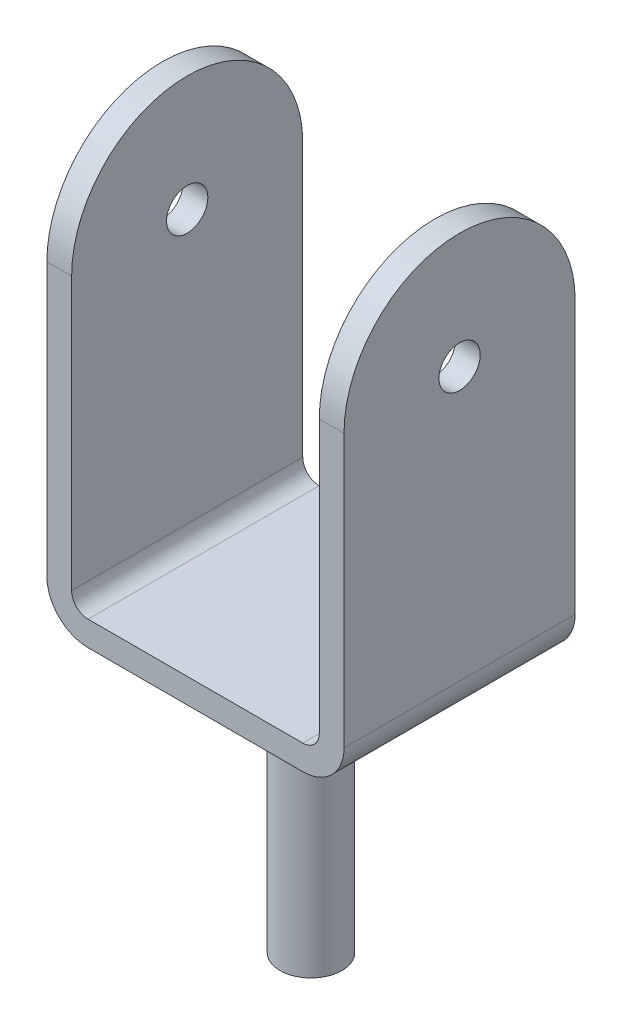
from build123d import *

# Parameters (mm, degrees)
U_CHANNEL_BODY_DEPTH     = 140
STEM_SKETCH_75_R         = 37.5
STEM_75_DEPTH            = 325
UPRIGHT_TOP_ROUNDS_R50_R = 50
CHANNEL_FILLETS_R20_R    = 20
SIDE_BOSS_SKETCH_R       = 140
SIDE_BOSS_DEPTH          = 30
PIN_HOLE_SKETCH_R        = 25
PIN_HOLES_DEPTH          = 648.765389628


with BuildPart() as part:
    # U-Channel Profile Sketch → U-Channel Body (new, symmetric)
    with BuildSketch(Plane.XY):
        Polygon((-180, 380), (-180, 0), (180, 0), (180, 380), (150, 380), (150, 30), (-150, 30), (-150, 380), align=None)
    extrude(amount=U_CHANNEL_BODY_DEPTH, both=True)

    # Stem Sketch Ø75 → Stem Ø75 (add)
    with BuildSketch(Plane.XZ):
        Circle(STEM_SKETCH_75_R)
    extrude(amount=STEM_75_DEPTH)

    # Upright Top Rounds R50
    upright_top_rounds_r50_edges = [part.edges().sort_by_distance(p)[0] for p in [
        (180, 0, 0),
        (-180, 0, 0),
    ]]
    fillet(upright_top_rounds_r50_edges, radius=UPRIGHT_TOP_ROUNDS_R50_R)

    # Channel Fillets R20
    channel_fillets_r20_edges = [part.edges().sort_by_distance(p)[0] for p in [
        (-150, 30, 0),
        (150, 30, 0),
    ]]
    fillet(channel_fillets_r20_edges, radius=CHANNEL_FILLETS_R20_R)

    # Side Boss Sketch → Side Boss (add)
    with BuildSketch(Plane(origin=(180, 0, 0), x_dir=(0, 0, -1), z_dir=(1, 0, 0))):
        with Locations((0, 380)):
            Circle(SIDE_BOSS_SKETCH_R)
    side_boss = extrude(amount=-SIDE_BOSS_DEPTH)

    # Side Boss Mirror: Side Boss across plane
    add(side_boss.mirror(Plane(origin=(0, 0, 0), x_dir=(0, 0, 1), z_dir=(1, 0, 0))))

    # Pin Hole Sketch → Pin Holes (cut, through all)
    with BuildSketch(Plane.ZY.offset(180)):
        with Locations(Location((0, 380, 0), (0, 0, 270))):
            Circle(PIN_HOLE_SKETCH_R)
    extrude(amount=-PIN_HOLES_DEPTH, mode=Mode.SUBTRACT)


solid = part.part
